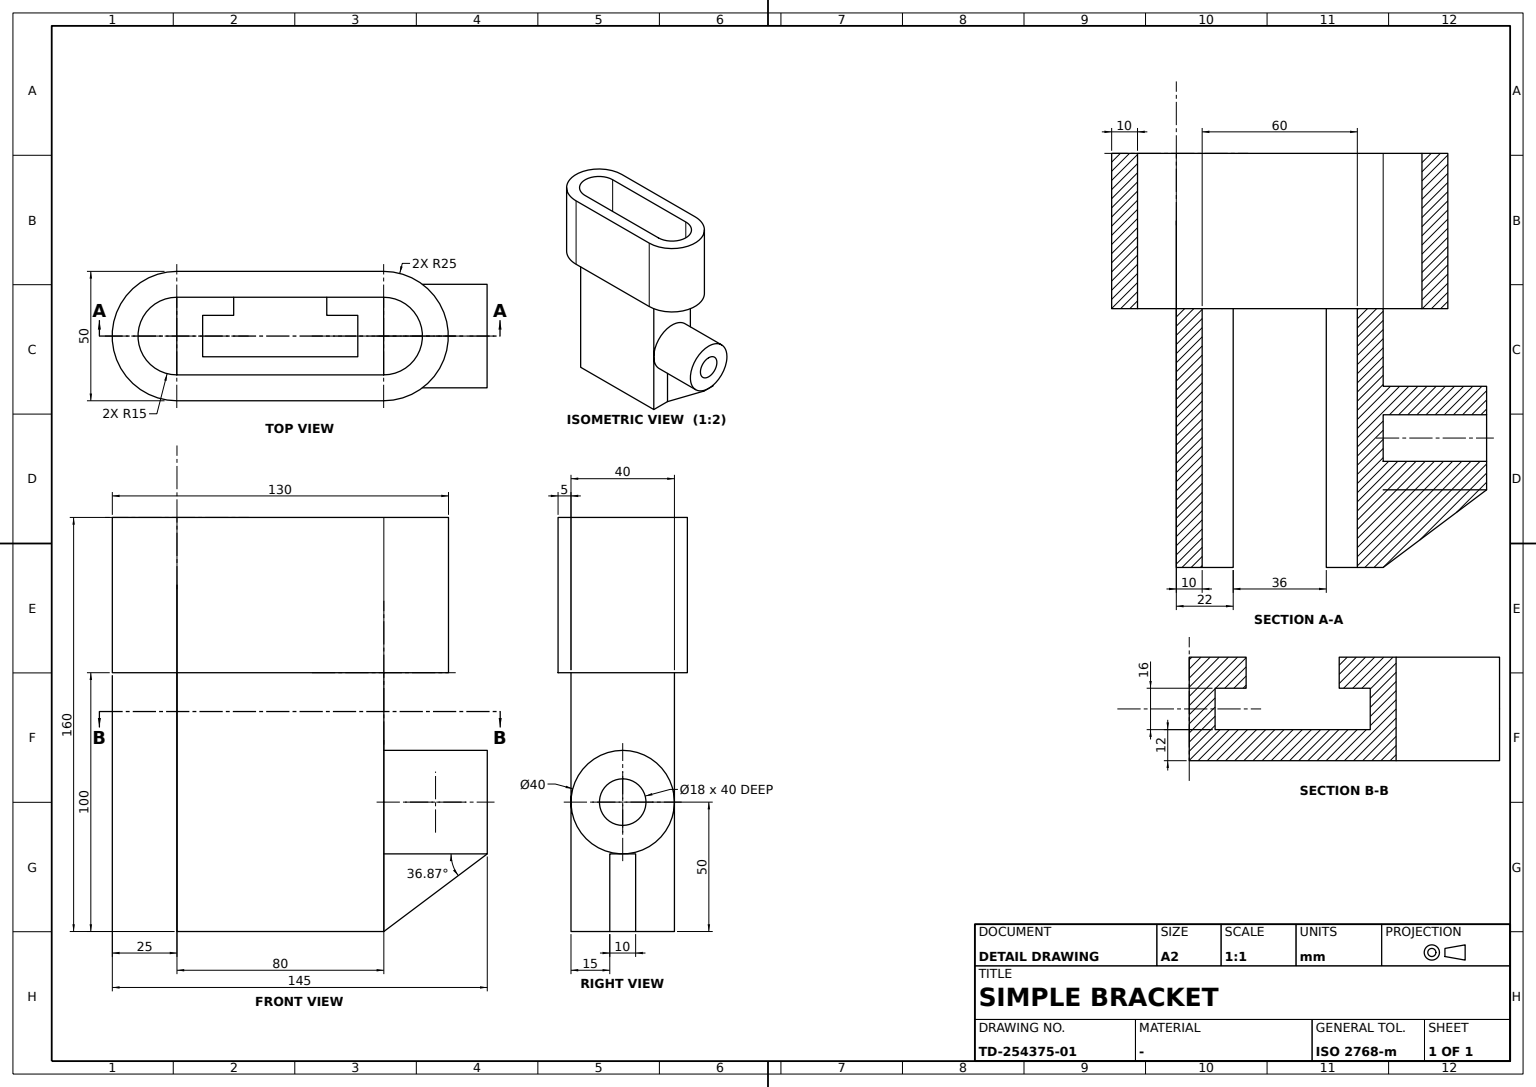
CATIA V5 part; units mm, degrees
sketch "Sketch1" plane through (0, 0, 0) normal (0, 0, 1) x (1, 0, 0)
  point P0 (-20, 0)
  line L0 (-20, 0) -> (20, 0)
  line L1 (20, 0) -> (20, -80)
  line L2 (20, -80) -> (-20, -80)
  line L3 (-20, -80) -> (-20, -58)
  line L4 (-20, -58) -> (-8, -58)
  line L5 (-8, -58) -> (-8, -70)
  line L6 (-8, -70) -> (8, -70)
  line L7 (8, -70) -> (8, -10)
  line L8 (8, -10) -> (-8, -10)
  point P1 (-8, -10)
  line L9 (-8, -10) -> (-8, -22)
  line L10 (-8, -22) -> (-20, -22)
  point P2 (-20, -22)
  line L11 (-20, -22) -> (-20, 0)
  dimension "distance L7 L1" = 12
  dimension "length L2" = 40
  dimension "length L1" = 80
  dimension "length L3" = 22
  dimension "length L5" = 12
  dimension "length L11" = 22
  dimension "length L9" = 12
  dimension "length L4" = 12
  constraint coincidence P0 x-axis
  constraint coincidence P1 L5
  constraint coincidence P2 L3
  constraint horizontal L0 x-axis
  constraint horizontal L2 x-axis
  constraint horizontal L4 x-axis
  constraint horizontal L6 x-axis
  constraint horizontal L8 x-axis
  constraint horizontal L10 x-axis
  constraint vertical L1 y-axis
  constraint vertical L3 y-axis
  constraint vertical L5 y-axis
  constraint vertical L7 y-axis
  constraint vertical L9 y-axis
  constraint vertical L11 y-axis
  constraint symmetry L11 L1 y-axis
extrude "Pad1" add sketch "Sketch1" along normal blind 100
sketch "Sketch2" plane through (0, 0, 0) normal (0, 1, 0) x (-1, 0, 0)
  circle A0 centre (0, 50) radius 9
  point P0 (0, 50)
  circle A1 centre (0, 50) radius 20
  line L0 (-20, 0) -> (20, 0) construction
  dimension "distance P0 L0" = 50
  dimension "radius A1" = 20
  dimension "radius A0" = 9
  constraint coincidence P0 y-axis
extrude "Pad2" add sketch "Sketch2" along normal blind 40
sketch "Sketch3" plane through (0, 0, 0) normal (1, 0, 0) x (0, 1, 0)
  line L0 (40, 30) -> (0, 30)
  point P0 (0, 30)
  line L1 (0, 30) -> (0, 0)
  line L2 (0, 0) -> (40, 30)
  constraint coincidence P0 y-axis
  constraint horizontal L0 x-axis
  constraint vertical L1 y-axis
extrude "Pad3" add sketch "Sketch3" along normal mid plane 10
sketch "Sketch4" plane through (0, 0, 100) normal (0, 0, 1) x (1, 0, 0)
  arc A0 (15, 0) -> (-15, 0) centre (0, 0) ccw
  arc A1 (-15, -80) -> (15, -80) centre (0, -80) ccw
  point P0 (0, -80)
  arc A2 (-25, -80) -> (25, -80) centre (0, -80) ccw
  arc A3 (25, 0) -> (-25, 0) centre (0, 0) ccw
  line L0 (-25, 0) -> (-25, -80)
  point P1 (-25, 0)
  line L1 (-15, 0) -> (-15, -80)
  point P2 (-15, 0)
  point P3 (-15, -80)
  line L2 (15, 0) -> (15, -80)
  point P4 (15, 0)
  point P5 (15, -80)
  line L3 (25, 0) -> (25, -80)
  point P6 (25, 0)
  point P7 (-15, -80)
  point P8 (15, -80)
  dimension "radius A0" = 15
  dimension "radius A3" = 25
  dimension "radius A1" = 15
  dimension "radius A2" = 25
  constraint coincidence P0 y-axis
  constraint coincidence P1 x-axis
  constraint coincidence P2 x-axis
  constraint coincidence P3 A1
  constraint coincidence P4 x-axis
  constraint coincidence P5 A1
  constraint coincidence P6 x-axis
  constraint coincidence L2 P8
  constraint coincidence L1 P7
  constraint coincidence P3 P7
  constraint coincidence P5 P8
  constraint vertical L0 y-axis
  constraint tangency L1 A1
  constraint tangency L2 A1
  constraint tangency L3 A2
extrude "Pad4" add sketch "Sketch4" along normal blind 60
